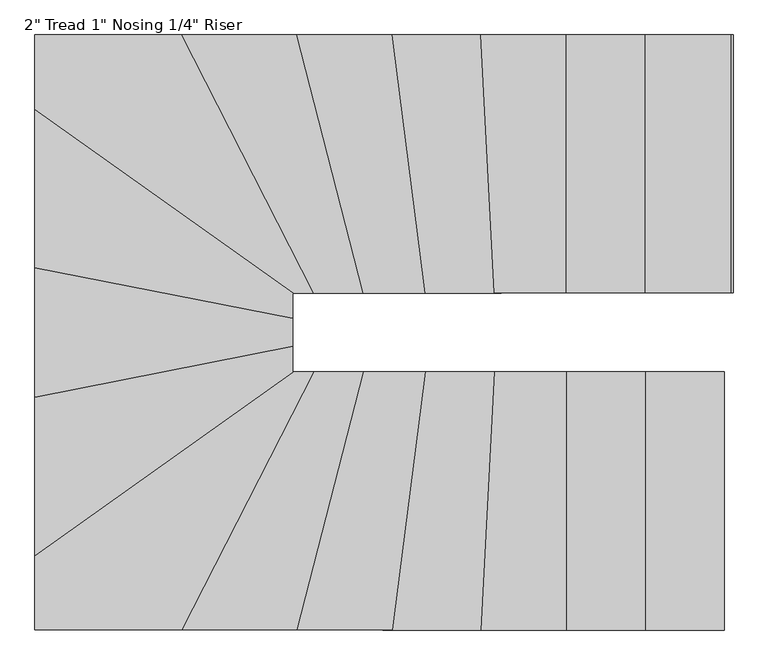
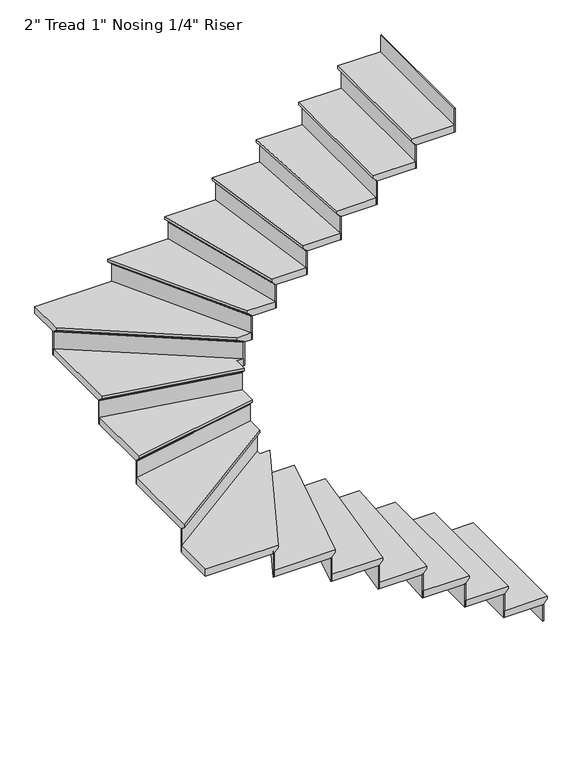
"""IFC4 building model written with IfcOpenShell, lengths in millimetres: stair flight geometry."""

from ifc_helpers import new_model, si_unit, origin, place, context, project, spatial, faceted_brep, source, transform, mapped, element, save


def stair_flight_257b0c60(model_context):
    return source(origin(), model_context, "Body", "Brep", [
        faceted_brep([(-7708.0614906, -9206.110779, 3510.2131579), (-7708.0614906, -9206.110779, 3529.2631579), (-7708.0614906, -10120.510779, 3529.2631579), (-7708.0614906, -10120.510779, 3510.2131579), (-7733.4614906, -9206.110779, 3484.8131579), (-7733.4614906, -10120.510779, 3484.8131579), (-8012.8614906, -9206.110779, 3529.2631579), (-8012.8614906, -10120.510779, 3529.2631579), (-7733.4614906, -10120.510779, 3478.4631579), (-8012.8614906, -10120.510779, 3478.4631579), (-8012.8614906, -9206.110779, 3478.4631579), (-7733.4614906, -9206.110779, 3478.4631579)], [[[0, 1, 2, 3]], [[4, 0, 3, 5]], [[2, 1, 6, 7]], [[8, 9, 10, 11]], [[2, 7, 9, 8, 5, 3]], [[8, 11, 4, 5]], [[6, 1, 0, 4, 11, 10]], [[7, 6, 10, 9]]]),
        faceted_brep([(-7733.4614906, -9206.110779, 3478.4631579), (-7733.4614906, -9206.110779, 3352.8), (-7739.8114906, -9206.110779, 3352.8), (-7739.8114906, -9206.110779, 3478.4631579), (-7733.4614906, -10120.510779, 3478.4631579), (-7739.8114906, -10120.510779, 3478.4631579), (-7739.8114906, -10120.510779, 3352.8), (-7733.4614906, -10120.510779, 3352.8)], [[[0, 1, 2, 3]], [[4, 5, 6, 7]], [[1, 0, 4, 7]], [[2, 1, 7, 6]], [[3, 2, 6, 5]], [[0, 3, 5, 4]]]),
        faceted_brep([(-8012.8614906, -9206.110779, 3654.9263158), (-8012.8614906, -9206.110779, 3478.4631579), (-8019.2114906, -9206.110779, 3478.4631579), (-8019.2114906, -9206.110779, 3654.9263158), (-8012.8614906, -10120.510779, 3654.9263158), (-8019.2114906, -10120.510779, 3654.9263158), (-8019.2114906, -10120.510779, 3478.4631579), (-8012.8614906, -10120.510779, 3478.4631579)], [[[0, 1, 2, 3]], [[4, 5, 6, 7]], [[1, 0, 4, 7]], [[2, 1, 7, 6]], [[3, 2, 6, 5]], [[0, 3, 5, 4]]]),
        faceted_brep([(-7987.4614906, -10120.510779, 3705.7263158), (-7987.4614906, -9206.110779, 3705.7263158), (-8292.2614906, -9206.110779, 3705.7263158), (-8292.2614906, -10120.510779, 3705.7263158), (-8012.8614906, -10120.510779, 3654.9263158), (-8292.2614906, -10120.510779, 3654.9263158), (-8292.2614906, -9206.110779, 3654.9263158), (-8012.8614906, -9206.110779, 3654.9263158), (-8012.8614906, -10120.510779, 3661.2763158), (-7987.4614906, -10120.510779, 3686.6763158), (-8012.8614906, -9206.110779, 3661.2763158), (-7987.4614906, -9206.110779, 3686.6763158)], [[[0, 1, 2, 3]], [[4, 5, 6, 7]], [[0, 3, 5, 4, 8, 9]], [[4, 7, 10, 8]], [[2, 1, 11, 10, 7, 6]], [[3, 2, 6, 5]], [[11, 1, 0, 9]], [[10, 11, 9, 8]]]),
        faceted_brep([(-8292.2614906, -9206.110779, 3831.3894737), (-8292.2614906, -9206.110779, 3654.9263158), (-8298.6114906, -9206.110779, 3654.9263158), (-8298.6114906, -9206.110779, 3831.3894737), (-8292.2614906, -10120.510779, 3831.3894737), (-8298.6114906, -10120.510779, 3831.3894737), (-8298.6114906, -10120.510779, 3654.9263158), (-8292.2614906, -10120.510779, 3654.9263158)], [[[0, 1, 2, 3]], [[4, 5, 6, 7]], [[1, 0, 4, 7]], [[2, 1, 7, 6]], [[3, 2, 6, 5]], [[0, 3, 5, 4]]]),
        faceted_brep([(-8266.8614906, -10120.510779, 3882.1894737), (-8266.8614906, -9206.110779, 3882.1894737), (-8547.928652, -9206.110779, 3882.1894737), (-8595.4629224, -10120.510779, 3882.1894737), (-8292.2614906, -10120.510779, 3831.3894737), (-8595.4629224, -10120.510779, 3831.3894737), (-8547.928652, -9206.110779, 3831.3894737), (-8292.2614906, -9206.110779, 3831.3894737), (-8292.2614906, -10120.510779, 3837.7394737), (-8266.8614906, -10120.510779, 3863.1394737), (-8292.2614906, -9206.110779, 3837.7394737), (-8266.8614906, -9206.110779, 3863.1394737)], [[[0, 1, 2, 3]], [[4, 5, 6, 7]], [[0, 3, 5, 4, 8, 9]], [[4, 7, 10, 8]], [[2, 1, 11, 10, 7, 6]], [[3, 2, 6, 5]], [[11, 1, 0, 9]], [[10, 11, 9, 8]]]),
        faceted_brep([(-8547.928652, -9206.110779, 4007.8526316), (-8547.928652, -9206.110779, 3831.3894737), (-8554.2872262, -9206.110779, 3831.3894737), (-8554.2872262, -9206.110779, 4007.8526316), (-8595.4629224, -10120.510779, 4007.8526316), (-8601.8214966, -10120.510779, 4007.8526316), (-8601.8214966, -10120.510779, 3831.3894737), (-8595.4629224, -10120.510779, 3831.3894737)], [[[0, 1, 2, 3]], [[4, 5, 6, 7]], [[1, 0, 4, 7]], [[2, 1, 7, 6]], [[3, 2, 6, 5]], [[0, 3, 5, 4]]]),
        faceted_brep([(-8570.0286258, -10120.510779, 4058.6526316), (-8522.4943554, -9206.110779, 4058.6526316), (-8792.0953519, -9206.110779, 4058.6526316), (-8910.4514035, -10120.510779, 4058.6526316), (-8595.4629224, -10120.510779, 4007.8526316), (-8910.4514035, -10120.510779, 4007.8526316), (-8792.0953519, -9206.110779, 4007.8526316), (-8547.928652, -9206.110779, 4007.8526316), (-8595.4629224, -10120.510779, 4014.2026316), (-8570.0286258, -10120.510779, 4039.6026316), (-8547.928652, -9206.110779, 4014.2026316), (-8522.4943554, -9206.110779, 4039.6026316)], [[[0, 1, 2, 3]], [[4, 5, 6, 7]], [[0, 3, 5, 4, 8, 9]], [[4, 7, 10, 8]], [[2, 1, 11, 10, 7, 6]], [[3, 2, 6, 5]], [[11, 1, 0, 9]], [[10, 11, 9, 8]]]),
        faceted_brep([(-8792.0953519, -9206.110779, 4184.3157895), (-8792.0953519, -9206.110779, 4007.8526316), (-8798.4983236, -9206.110779, 4007.8526316), (-8798.4983236, -9206.110779, 4184.3157895), (-8910.4514035, -10120.510779, 4184.3157895), (-8916.8543753, -10120.510779, 4184.3157895), (-8916.8543753, -10120.510779, 4007.8526316), (-8910.4514035, -10120.510779, 4007.8526316)], [[[0, 1, 2, 3]], [[4, 5, 6, 7]], [[1, 0, 4, 7]], [[2, 1, 7, 6]], [[3, 2, 6, 5]], [[0, 3, 5, 4]]]),
        faceted_brep([(-8884.8395164, -10120.510779, 4235.1157895), (-8766.4834647, -9206.110779, 4235.1157895), (-9013.7225743, -9206.110779, 4235.1157895), (-9248.8530217, -10120.510779, 4235.1157895), (-8910.4514035, -10120.510779, 4184.3157895), (-9248.8530217, -10120.510779, 4184.3157895), (-9013.7225743, -9206.110779, 4184.3157895), (-8792.0953519, -9206.110779, 4184.3157895), (-8910.4514035, -10120.510779, 4190.6657895), (-8884.8395164, -10120.510779, 4216.0657895), (-8792.0953519, -9206.110779, 4190.6657895), (-8766.4834647, -9206.110779, 4216.0657895)], [[[0, 1, 2, 3]], [[4, 5, 6, 7]], [[0, 3, 5, 4, 8, 9]], [[4, 7, 10, 8]], [[2, 1, 11, 10, 7, 6]], [[3, 2, 6, 5]], [[11, 1, 0, 9]], [[10, 11, 9, 8]]]),
        faceted_brep([(-9013.7225743, -9206.110779, 4360.7789474), (-9013.7225743, -9206.110779, 4184.3157895), (-9020.2791512, -9206.110779, 4184.3157895), (-9020.2791512, -9206.110779, 4360.7789474), (-9248.8530217, -10120.510779, 4360.7789474), (-9255.4095986, -10120.510779, 4360.7789474), (-9255.4095986, -10120.510779, 4184.3157895), (-9248.8530217, -10120.510779, 4184.3157895)], [[[0, 1, 2, 3]], [[4, 5, 6, 7]], [[1, 0, 4, 7]], [[2, 1, 7, 6]], [[3, 2, 6, 5]], [[0, 3, 5, 4]]]),
        faceted_brep([(-9222.6267143, -10120.510779, 4411.5789474), (-8987.4962669, -9206.110779, 4411.5789474), (-9190.0692104, -9206.110779, 4411.5789474), (-9658.8938317, -10120.510779, 4411.5789474), (-9248.8530217, -10120.510779, 4360.7789474), (-9658.8938317, -10120.510779, 4360.7789474), (-9190.0692104, -9206.110779, 4360.7789474), (-9013.7225743, -9206.110779, 4360.7789474), (-9248.8530217, -10120.510779, 4367.1289474), (-9222.6267143, -10120.510779, 4392.5289474), (-9013.7225743, -9206.110779, 4367.1289474), (-8987.4962669, -9206.110779, 4392.5289474)], [[[0, 1, 2, 3]], [[4, 5, 6, 7]], [[0, 3, 5, 4, 8, 9]], [[4, 7, 10, 8]], [[2, 1, 11, 10, 7, 6]], [[3, 2, 6, 5]], [[11, 1, 0, 9]], [[10, 11, 9, 8]]]),
        faceted_brep([(-9190.0692104, -9206.110779, 4537.2421053), (-9190.0692104, -9206.110779, 4360.7789474), (-9197.2051936, -9206.110779, 4360.7789474), (-9197.2051936, -9206.110779, 4537.2421053), (-9658.8938317, -10120.510779, 4537.2421053), (-9666.0298149, -10120.510779, 4537.2421053), (-9666.0298149, -10120.510779, 4360.7789474), (-9658.8938317, -10120.510779, 4360.7789474)], [[[0, 1, 2, 3]], [[4, 5, 6, 7]], [[1, 0, 4, 7]], [[2, 1, 7, 6]], [[3, 2, 6, 5]], [[0, 3, 5, 4]]]),
        faceted_brep([(-10150.1931824, -9826.8296453, 4588.0421053), (-10150.1931824, -10120.510779, 4588.0421053), (-9630.3498992, -10120.510779, 4588.0421053), (-9161.5252779, -9206.110779, 4588.0421053), (-9235.7931824, -9206.110779, 4588.0421053), (-9235.7931824, -9176.5556961, 4588.0421053), (-10150.1931824, -10120.510779, 4537.2421053), (-10150.1931824, -9826.8296453, 4537.2421053), (-9235.7931824, -9176.5556961, 4537.2421053), (-9235.7931824, -9206.110779, 4537.2421053), (-9190.0692104, -9206.110779, 4537.2421053), (-9658.8938317, -10120.510779, 4537.2421053), (-9658.8938317, -10120.510779, 4543.5921053), (-9630.3498992, -10120.510779, 4568.9921053), (-9190.0692104, -9206.110779, 4543.5921053), (-9161.5252779, -9206.110779, 4568.9921053)], [[[0, 1, 2, 3, 4, 5]], [[6, 7, 8, 9, 10, 11]], [[1, 0, 7, 6]], [[2, 1, 6, 11, 12, 13]], [[11, 10, 14, 12]], [[4, 3, 15, 14, 10, 9]], [[5, 4, 9, 8]], [[0, 5, 8, 7]], [[15, 3, 2, 13]], [[14, 15, 13, 12]]]),
        faceted_brep([(-9235.7931824, -9176.5556961, 4713.7052632), (-9235.7931824, -9176.5556961, 4537.2421053), (-9235.7931824, -9168.7637213, 4537.2421053), (-9235.7931824, -9168.7637213, 4713.7052632), (-10150.1931824, -9826.8296453, 4713.7052632), (-10150.1931824, -9819.0376705, 4713.7052632), (-10150.1931824, -9819.0376705, 4537.2421053), (-10150.1931824, -9826.8296453, 4537.2421053)], [[[0, 1, 2, 3]], [[4, 5, 6, 7]], [[1, 0, 4, 7]], [[2, 1, 7, 6]], [[3, 2, 6, 5]], [[0, 3, 5, 4]]]),
        faceted_brep([(-10150.1931824, -9857.9975445, 4764.5052632), (-9235.7931824, -9207.7235953, 4764.5052632), (-9235.7931824, -9090.1016091, 4764.5052632), (-10150.1931824, -9270.3424654, 4764.5052632), (-10150.1931824, -9826.8296453, 4713.7052632), (-10150.1931824, -9270.3424654, 4713.7052632), (-9235.7931824, -9090.1016091, 4713.7052632), (-9235.7931824, -9176.5556961, 4713.7052632), (-10150.1931824, -9826.8296453, 4720.0552632), (-10150.1931824, -9857.9975445, 4745.4552632), (-9235.7931824, -9176.5556961, 4720.0552632), (-9235.7931824, -9207.7235953, 4745.4552632)], [[[0, 1, 2, 3]], [[4, 5, 6, 7]], [[0, 3, 5, 4, 8, 9]], [[4, 7, 10, 8]], [[2, 1, 11, 10, 7, 6]], [[3, 2, 6, 5]], [[11, 1, 0, 9]], [[10, 11, 9, 8]]]),
        faceted_brep([(-9235.7931824, -9090.1016091, 4890.1684211), (-9235.7931824, -9090.1016091, 4713.7052632), (-9235.7931824, -9083.6294236, 4713.7052632), (-9235.7931824, -9083.6294236, 4890.1684211), (-10150.1931824, -9270.3424654, 4890.1684211), (-10150.1931824, -9263.87028, 4890.1684211), (-10150.1931824, -9263.87028, 4713.7052632), (-10150.1931824, -9270.3424654, 4713.7052632)], [[[0, 1, 2, 3]], [[4, 5, 6, 7]], [[1, 0, 4, 7]], [[2, 1, 7, 6]], [[3, 2, 6, 5]], [[0, 3, 5, 4]]]),
        faceted_brep([(-10150.1931824, -9296.2312071, 4940.9684211), (-9235.7931824, -9115.9903508, 4940.9684211), (-9235.7931824, -8990.9424654, 4940.9684211), (-10150.1931824, -8810.7016091, 4940.9684211), (-10150.1931824, -9270.3424654, 4890.1684211), (-10150.1931824, -8810.7016091, 4890.1684211), (-9235.7931824, -8990.9424654, 4890.1684211), (-9235.7931824, -9090.1016091, 4890.1684211), (-10150.1931824, -9270.3424654, 4896.5184211), (-10150.1931824, -9296.2312071, 4921.9184211), (-9235.7931824, -9090.1016091, 4896.5184211), (-9235.7931824, -9115.9903508, 4921.9184211)], [[[0, 1, 2, 3]], [[4, 5, 6, 7]], [[0, 3, 5, 4, 8, 9]], [[4, 7, 10, 8]], [[2, 1, 11, 10, 7, 6]], [[3, 2, 6, 5]], [[11, 1, 0, 9]], [[10, 11, 9, 8]]]),
        faceted_brep([(-9235.7931824, -8990.9424654, 5066.6315789), (-9235.7931824, -8990.9424654, 4890.1684211), (-9235.7931824, -8984.47028, 4890.1684211), (-9235.7931824, -8984.47028, 5066.6315789), (-10150.1931824, -8810.7016091, 5066.6315789), (-10150.1931824, -8804.2294236, 5066.6315789), (-10150.1931824, -8804.2294236, 4890.1684211), (-10150.1931824, -8810.7016091, 4890.1684211)], [[[0, 1, 2, 3]], [[4, 5, 6, 7]], [[1, 0, 4, 7]], [[2, 1, 7, 6]], [[3, 2, 6, 5]], [[0, 3, 5, 4]]]),
        faceted_brep([(-10150.1931824, -8836.5903508, 5117.4315789), (-9235.7931824, -9016.8312071, 5117.4315789), (-9235.7931824, -8926.710779, 5117.4315789), (-9189.6977079, -8926.710779, 5117.4315789), (-10150.1931824, -8243.6561143, 5117.4315789), (-10150.1931824, -8810.7016091, 5066.6315789), (-10150.1931824, -8243.6561143, 5066.6315789), (-9189.6977079, -8926.710779, 5066.6315789), (-9235.7931824, -8926.710779, 5066.6315789), (-9235.7931824, -8990.9424654, 5066.6315789), (-10150.1931824, -8810.7016091, 5072.9815789), (-10150.1931824, -8836.5903508, 5098.3815789), (-9235.7931824, -8990.9424654, 5072.9815789), (-9235.7931824, -9016.8312071, 5098.3815789)], [[[0, 1, 2, 3, 4]], [[5, 6, 7, 8, 9]], [[0, 4, 6, 5, 10, 11]], [[5, 9, 12, 10]], [[2, 1, 13, 12, 9, 8]], [[3, 2, 8, 7]], [[4, 3, 7, 6]], [[13, 1, 0, 11]], [[12, 13, 11, 10]]]),
        faceted_brep([(-9189.6977079, -8926.710779, 5243.0947368), (-9189.6977079, -8926.710779, 5066.6315789), (-9178.7408154, -8926.710779, 5066.6315789), (-9178.7408154, -8926.710779, 5243.0947368), (-10150.1931824, -8243.6561143, 5243.0947368), (-10150.1931824, -8235.8641395, 5243.0947368), (-10150.1931824, -8235.8641395, 5066.6315789), (-10150.1931824, -8243.6561143, 5066.6315789)], [[[0, 1, 2, 3]], [[4, 5, 6, 7]], [[1, 0, 4, 7]], [[2, 1, 7, 6]], [[3, 2, 6, 5]], [[0, 3, 5, 4]]]),
        faceted_brep([(-9601.8059667, -8012.310779, 5293.8947368), (-10150.1931824, -8012.310779, 5293.8947368), (-10150.1931824, -8274.8240135, 5293.8947368), (-9233.5252779, -8926.710779, 5293.8947368), (-9132.9813454, -8926.710779, 5293.8947368), (-10150.1931824, -8012.310779, 5243.0947368), (-9601.8059667, -8012.310779, 5243.0947368), (-9132.9813454, -8926.710779, 5243.0947368), (-9189.6977079, -8926.710779, 5243.0947368), (-10150.1931824, -8243.6561143, 5243.0947368), (-10150.1931824, -8243.6561143, 5249.4447368), (-10150.1931824, -8274.8240135, 5274.8447368), (-9189.6977079, -8926.710779, 5249.4447368), (-9233.5252779, -8926.710779, 5274.8447368)], [[[0, 1, 2, 3, 4]], [[5, 6, 7, 8, 9]], [[1, 0, 6, 5]], [[2, 1, 5, 9, 10, 11]], [[9, 8, 12, 10]], [[4, 3, 13, 12, 8, 7]], [[0, 4, 7, 6]], [[13, 3, 2, 11]], [[12, 13, 11, 10]]]),
        faceted_brep([(-9132.9813454, -8926.710779, 5419.5578947), (-9132.9813454, -8926.710779, 5243.0947368), (-9125.8453622, -8926.710779, 5243.0947368), (-9125.8453622, -8926.710779, 5419.5578947), (-9601.8059667, -8012.310779, 5419.5578947), (-9594.6699835, -8012.310779, 5419.5578947), (-9594.6699835, -8012.310779, 5243.0947368), (-9601.8059667, -8012.310779, 5243.0947368)], [[[0, 1, 2, 3]], [[4, 5, 6, 7]], [[1, 0, 4, 7]], [[2, 1, 7, 6]], [[3, 2, 6, 5]], [[0, 3, 5, 4]]]),
        faceted_brep([(-9630.3498992, -8012.310779, 5470.3578947), (-9161.5252779, -8926.710779, 5470.3578947), (-8961.2699594, -8926.710779, 5470.3578947), (-9196.4004068, -8012.310779, 5470.3578947), (-9601.8059667, -8012.310779, 5419.5578947), (-9196.4004068, -8012.310779, 5419.5578947), (-8961.2699594, -8926.710779, 5419.5578947), (-9132.9813454, -8926.710779, 5419.5578947), (-9601.8059667, -8012.310779, 5425.9078947), (-9630.3498992, -8012.310779, 5451.3078947), (-9132.9813454, -8926.710779, 5425.9078947), (-9161.5252779, -8926.710779, 5451.3078947)], [[[0, 1, 2, 3]], [[4, 5, 6, 7]], [[0, 3, 5, 4, 8, 9]], [[4, 7, 10, 8]], [[2, 1, 11, 10, 7, 6]], [[3, 2, 6, 5]], [[11, 1, 0, 9]], [[10, 11, 9, 8]]]),
        faceted_brep([(-8961.2699594, -8926.710779, 5596.0210526), (-8961.2699594, -8926.710779, 5419.5578947), (-8954.7133825, -8926.710779, 5419.5578947), (-8954.7133825, -8926.710779, 5596.0210526), (-9196.4004068, -8012.310779, 5596.0210526), (-9189.84383, -8012.310779, 5596.0210526), (-9189.84383, -8012.310779, 5419.5578947), (-9196.4004068, -8012.310779, 5419.5578947)], [[[0, 1, 2, 3]], [[4, 5, 6, 7]], [[1, 0, 4, 7]], [[2, 1, 7, 6]], [[3, 2, 6, 5]], [[0, 3, 5, 4]]]),
        faceted_brep([(-9222.6267143, -8012.310779, 5646.8210526), (-8987.4962669, -8926.710779, 5646.8210526), (-8740.8715776, -8926.710779, 5646.8210526), (-8859.2276293, -8012.310779, 5646.8210526), (-9196.4004068, -8012.310779, 5596.0210526), (-8859.2276293, -8012.310779, 5596.0210526), (-8740.8715776, -8926.710779, 5596.0210526), (-8961.2699594, -8926.710779, 5596.0210526), (-9196.4004068, -8012.310779, 5602.3710526), (-9222.6267143, -8012.310779, 5627.7710526), (-8961.2699594, -8926.710779, 5602.3710526), (-8987.4962669, -8926.710779, 5627.7710526)], [[[0, 1, 2, 3]], [[4, 5, 6, 7]], [[0, 3, 5, 4, 8, 9]], [[4, 7, 10, 8]], [[2, 1, 11, 10, 7, 6]], [[3, 2, 6, 5]], [[11, 1, 0, 9]], [[10, 11, 9, 8]]]),
        faceted_brep([(-8740.8715776, -8926.710779, 5772.4842105), (-8740.8715776, -8926.710779, 5596.0210526), (-8734.4686059, -8926.710779, 5596.0210526), (-8734.4686059, -8926.710779, 5772.4842105), (-8859.2276293, -8012.310779, 5772.4842105), (-8852.8246575, -8012.310779, 5772.4842105), (-8852.8246575, -8012.310779, 5596.0210526), (-8859.2276293, -8012.310779, 5596.0210526)], [[[0, 1, 2, 3]], [[4, 5, 6, 7]], [[1, 0, 4, 7]], [[2, 1, 7, 6]], [[3, 2, 6, 5]], [[0, 3, 5, 4]]]),
        faceted_brep([(-8884.8395164, -8012.310779, 5823.2842105), (-8766.4834647, -8926.710779, 5823.2842105), (-8497.0600587, -8926.710779, 5823.2842105), (-8544.5943291, -8012.310779, 5823.2842105), (-8859.2276293, -8012.310779, 5772.4842105), (-8544.5943291, -8012.310779, 5772.4842105), (-8497.0600587, -8926.710779, 5772.4842105), (-8740.8715776, -8926.710779, 5772.4842105), (-8859.2276293, -8012.310779, 5778.8342105), (-8884.8395164, -8012.310779, 5804.2342105), (-8740.8715776, -8926.710779, 5778.8342105), (-8766.4834647, -8926.710779, 5804.2342105)], [[[0, 1, 2, 3]], [[4, 5, 6, 7]], [[0, 3, 5, 4, 8, 9]], [[4, 7, 10, 8]], [[2, 1, 11, 10, 7, 6]], [[3, 2, 6, 5]], [[11, 1, 0, 9]], [[10, 11, 9, 8]]]),
        faceted_brep([(-8497.0600587, -8926.710779, 5948.9473684), (-8497.0600587, -8926.710779, 5772.4842105), (-8490.7014845, -8926.710779, 5772.4842105), (-8490.7014845, -8926.710779, 5948.9473684), (-8544.5943291, -8012.310779, 5948.9473684), (-8538.235755, -8012.310779, 5948.9473684), (-8538.235755, -8012.310779, 5772.4842105), (-8544.5943291, -8012.310779, 5772.4842105)], [[[0, 1, 2, 3]], [[4, 5, 6, 7]], [[1, 0, 4, 7]], [[2, 1, 7, 6]], [[3, 2, 6, 5]], [[0, 3, 5, 4]]]),
        faceted_brep([(-8570.0286258, -8012.310779, 5999.7473684), (-8522.4943554, -8926.710779, 5999.7473684), (-8241.4614906, -8926.710779, 5999.7473684), (-8241.4614906, -8012.310779, 5999.7473684), (-8544.5943291, -8012.310779, 5948.9473684), (-8241.4614906, -8012.310779, 5948.9473684), (-8241.4614906, -8926.710779, 5948.9473684), (-8497.0600587, -8926.710779, 5948.9473684), (-8544.5943291, -8012.310779, 5955.2973684), (-8570.0286258, -8012.310779, 5980.6973684), (-8497.0600587, -8926.710779, 5955.2973684), (-8522.4943554, -8926.710779, 5980.6973684)], [[[0, 1, 2, 3]], [[4, 5, 6, 7]], [[0, 3, 5, 4, 8, 9]], [[4, 7, 10, 8]], [[2, 1, 11, 10, 7, 6]], [[3, 2, 6, 5]], [[11, 1, 0, 9]], [[10, 11, 9, 8]]]),
        faceted_brep([(-8241.4614906, -8926.710779, 6125.4105263), (-8241.4614906, -8926.710779, 5948.9473684), (-8235.1114906, -8926.710779, 5948.9473684), (-8235.1114906, -8926.710779, 6125.4105263), (-8241.4614906, -8012.310779, 6125.4105263), (-8235.1114906, -8012.310779, 6125.4105263), (-8235.1114906, -8012.310779, 5948.9473684), (-8241.4614906, -8012.310779, 5948.9473684)], [[[0, 1, 2, 3]], [[4, 5, 6, 7]], [[1, 0, 4, 7]], [[2, 1, 7, 6]], [[3, 2, 6, 5]], [[0, 3, 5, 4]]]),
        faceted_brep([(-8266.8614906, -8012.310779, 6176.2105263), (-8266.8614906, -8926.710779, 6176.2105263), (-7962.0614906, -8926.710779, 6176.2105263), (-7962.0614906, -8012.310779, 6176.2105263), (-8241.4614906, -8012.310779, 6125.4105263), (-7962.0614906, -8012.310779, 6125.4105263), (-7962.0614906, -8926.710779, 6125.4105263), (-8241.4614906, -8926.710779, 6125.4105263), (-8241.4614906, -8012.310779, 6131.7605263), (-8266.8614906, -8012.310779, 6157.1605263), (-8241.4614906, -8926.710779, 6131.7605263), (-8266.8614906, -8926.710779, 6157.1605263)], [[[0, 1, 2, 3]], [[4, 5, 6, 7]], [[0, 3, 5, 4, 8, 9]], [[4, 7, 10, 8]], [[2, 1, 11, 10, 7, 6]], [[3, 2, 6, 5]], [[11, 1, 0, 9]], [[10, 11, 9, 8]]]),
        faceted_brep([(-7962.0614906, -8926.710779, 6301.8736842), (-7962.0614906, -8926.710779, 6125.4105263), (-7955.7114906, -8926.710779, 6125.4105263), (-7955.7114906, -8926.710779, 6301.8736842), (-7962.0614906, -8012.310779, 6301.8736842), (-7955.7114906, -8012.310779, 6301.8736842), (-7955.7114906, -8012.310779, 6125.4105263), (-7962.0614906, -8012.310779, 6125.4105263)], [[[0, 1, 2, 3]], [[4, 5, 6, 7]], [[1, 0, 4, 7]], [[2, 1, 7, 6]], [[3, 2, 6, 5]], [[0, 3, 5, 4]]]),
        faceted_brep([(-7682.6614906, -8926.710779, 6478.3368421), (-7682.6614906, -8926.710779, 6301.8736842), (-7676.3114906, -8926.710779, 6301.8736842), (-7676.3114906, -8926.710779, 6478.3368421), (-7682.6614906, -8012.310779, 6478.3368421), (-7676.3114906, -8012.310779, 6478.3368421), (-7676.3114906, -8012.310779, 6301.8736842), (-7682.6614906, -8012.310779, 6301.8736842)], [[[0, 1, 2, 3]], [[4, 5, 6, 7]], [[1, 0, 4, 7]], [[2, 1, 7, 6]], [[3, 2, 6, 5]], [[0, 3, 5, 4]]]),
        faceted_brep([(-7987.4614906, -8012.310779, 6352.6736842), (-7987.4614906, -8926.710779, 6352.6736842), (-7682.6614906, -8926.710779, 6352.6736842), (-7682.6614906, -8012.310779, 6352.6736842), (-7962.0614906, -8012.310779, 6301.8736842), (-7682.6614906, -8012.310779, 6301.8736842), (-7682.6614906, -8926.710779, 6301.8736842), (-7962.0614906, -8926.710779, 6301.8736842), (-7962.0614906, -8012.310779, 6308.2236842), (-7987.4614906, -8012.310779, 6333.6236842), (-7962.0614906, -8926.710779, 6308.2236842), (-7987.4614906, -8926.710779, 6333.6236842)], [[[0, 1, 2, 3]], [[4, 5, 6, 7]], [[0, 3, 5, 4, 8, 9]], [[4, 7, 10, 8]], [[2, 1, 11, 10, 7, 6]], [[3, 2, 6, 5]], [[11, 1, 0, 9]], [[10, 11, 9, 8]]]),
    ])


if __name__ == "__main__":
    model = new_model("IFC4")
    model_context = context("Model", 3, world=origin())
    ifc_project = project(units=[si_unit("LENGTHUNIT", "METRE", prefix="MILLI")], contexts=[model_context])
    site = spatial("IfcSite", under=ifc_project)
    building = spatial("IfcBuilding", under=site)
    placement = place(None, origin())
    stair_flight_shape = stair_flight_257b0c60(model_context)
    element("IfcStairFlight", 1, ObjectType="2\" Tread 1\" Nosing 1/4\" Riser", at=placement, inside=building, context=model_context, shape_type="MappedRepresentation", body=[
        mapped(stair_flight_shape, transform((0.0, 0.0, 0.0), x_axis=(1.0, 0.0, 0.0), y_axis=(0.0, 1.0, 0.0), z_axis=(0.0, 0.0, 1.0))),
    ])
    save(model, "model.ifc")
